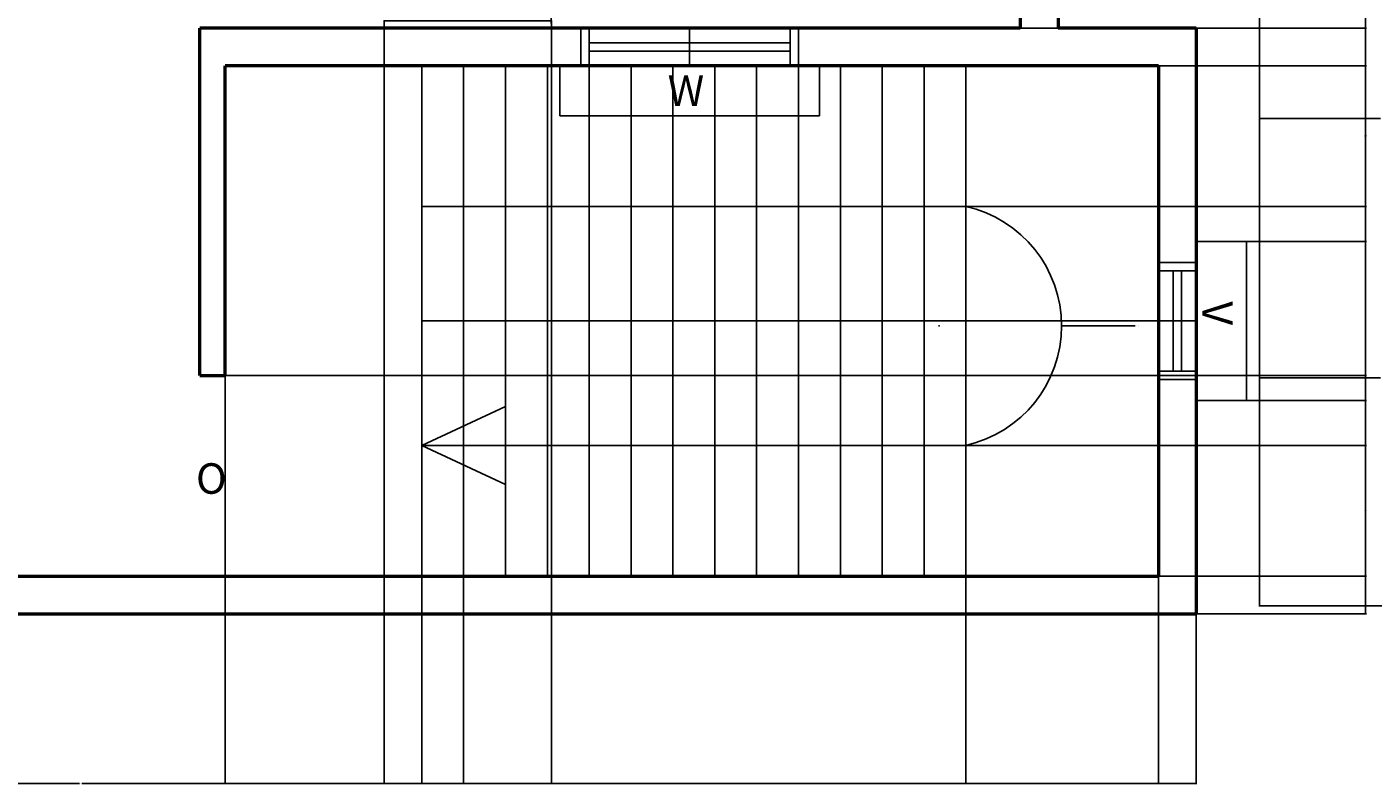
# Model space of a CAD drawing. Units: inches. Extents: x -73 to 1162, y -188 to 590.
# Tile 4 of 9: x 222 to 543, y -188 to -8. Entities that reach past the tile are written whole.
import ezdxf

# ---------------------------------------------------------------- set-up
doc = ezdxf.new("R2010")
doc.units = ezdxf.units.IN
doc.header["$MEASUREMENT"] = 0
for name, color, linetype, lineweight in [('A-ANNO-DIMS', 2, 'Continuous', 18), ('A-ANNO-TEXT', 7, 'Continuous', 25), ('A-DOOR', 3, 'Continuous', 25), ('A-FLOR-STRS', 3, 'Continuous', 25), ('A-GLAZ', 4, 'Continuous', 25), ('A-WALL', 7, 'Continuous', 50)]:
    doc.layers.add(name, color=color, linetype=linetype, lineweight=lineweight)
doc.styles.get("Standard").update_dxf_attribs({"font": 'arial.ttf'})
doc.dimstyles.get("Standard").update_dxf_attribs({"dimtxt": 0.18, "dimasz": 0.18, "dimexe": 0.18, "dimexo": 0.0625, "dimgap": 0.09, "dimtad": 0, "dimtih": 1, "dimtoh": 1, "dimdec": 1, "dimzin": 0, "dimdsep": 46, "dimlunit": 4, "dimtxsty": 'Standard', "dimcen": 0.09, "dimadec": 0, "dimazin": 0, "dimtfac": 1, "dimtdec": 1, "dimtofl": 0, "dimtmove": 0, "dimatfit": 3, "dimfxl": 1, "dimtolj": 1, "dimtzin": 0, "dimarcsym": 0})

# ---------------------------------------------------------------- blocks, each defined once
blk = doc.blocks.new('*U7')
for p, q in [((0, 0), (0, 6)), ((40, 0), (40, 6))]:
    blk.add_line(p, q)
blk.add_lwpolyline([(0, 0), (0, -40), (1.75, -40), (1.75, 0)], close=True)
blk.add_arc((0, 0), 40, 270, 360)
blk = doc.blocks.new('VENT-V')
for p, q in [((0, 9), (0, 21)), ((38, 21), (0, 21)), ((38, 9), (38, 21)), ((5, 9), (0, 9)), ((5, 0), (5, 9)), ((33, 0), (33, 9)), ((33, 9), (38, 9))]:
    blk.add_line(p, q)
blk = doc.blocks.new('*D58')
at = {"layer": 'A-ANNO-DIMS', "color": 0, "lineweight": -2, "transparency": 16777216}
for p, q in [((-31.83, -147.88), (-31.83, -188.5)), ((501.17, -147.88), (501.17, -188.5)), ((-31.65, -188.32), (234.38, -188.32)), ((500.99, -188.32), (234.96, -188.32))]:
    blk.add_line(p, q, dxfattribs=at)
at = {"layer": 'A-ANNO-DIMS', "color": 0, "transparency": 16777216}
for points in [[(-31.65, -188.29), (-31.65, -188.35), (-31.83, -188.32)], [(500.99, -188.29), (500.99, -188.35), (501.17, -188.32)]]:
    blk.add_solid(points, dxfattribs=at)
at = {"layer": 'Defpoints', "color": 0, "transparency": 16777216}
for p in [(-31.83, -147.82), (501.17, -147.82), (501.17, -188.32)]:
    blk.add_point(p, dxfattribs=at)
at = {"layer": 'A-ANNO-DIMS', "color": 0, "transparency": 16777216, "insert": (234.67, -188.32), "char_height": 0.18, "attachment_point": 5}
blk.add_mtext('\\A1;533', dxfattribs=at)
blk = doc.blocks.new('*D74')
at = {"layer": 'A-ANNO-DIMS', "color": 0, "lineweight": -2, "transparency": 16777216}
for p, q in [((480.23, 36.68), (541.85, 36.68)), ((541.67, 36.5), (541.67, 14.62)), ((541.67, -7.64), (541.67, 14.25)), ((501.23, -7.82), (541.85, -7.82))]:
    blk.add_line(p, q, dxfattribs=at)
at = {"layer": 'A-ANNO-DIMS', "color": 0, "transparency": 16777216}
for points in [[(541.64, 36.5), (541.7, 36.5), (541.67, 36.68)], [(541.64, -7.64), (541.7, -7.64), (541.67, -7.82)]]:
    blk.add_solid(points, dxfattribs=at)
at = {"layer": 'Defpoints', "color": 0, "transparency": 16777216}
for p in [(480.17, 36.68), (501.17, -7.82), (541.67, -7.82)]:
    blk.add_point(p, dxfattribs=at)
at = {"layer": 'A-ANNO-DIMS', "color": 0, "transparency": 16777216, "insert": (541.67, 14.43), "char_height": 0.18, "attachment_point": 5}
blk.add_mtext('\\A1;44.5', dxfattribs=at)
blk = doc.blocks.new('*D75')
at = {"layer": 'A-ANNO-DIMS', "color": 0, "lineweight": -2, "transparency": 16777216}
for p, q in [((501.23, -7.82), (541.85, -7.82)), ((541.67, -8), (541.67, -33.13)), ((541.67, -58.64), (541.67, -33.5)), ((501.23, -58.82), (541.85, -58.82))]:
    blk.add_line(p, q, dxfattribs=at)
at = {"layer": 'A-ANNO-DIMS', "color": 0, "transparency": 16777216}
for points in [[(541.64, -8), (541.7, -8), (541.67, -7.82)], [(541.64, -58.64), (541.7, -58.64), (541.67, -58.82)]]:
    blk.add_solid(points, dxfattribs=at)
at = {"layer": 'Defpoints', "color": 0, "transparency": 16777216}
for p in [(501.17, -7.82), (501.17, -58.82), (541.67, -58.82)]:
    blk.add_point(p, dxfattribs=at)
at = {"layer": 'A-ANNO-DIMS', "color": 0, "transparency": 16777216, "insert": (541.67, -33.32), "char_height": 0.18, "attachment_point": 5}
blk.add_mtext('\\A1;51', dxfattribs=at)
blk = doc.blocks.new('*D76')
at = {"layer": 'A-ANNO-DIMS', "color": 0, "lineweight": -2, "transparency": 16777216}
for p, q in [((501.23, -96.82), (541.85, -96.82)), ((541.67, -97), (541.67, -122.13)), ((541.67, -147.64), (541.67, -122.5)), ((501.23, -147.82), (541.85, -147.82))]:
    blk.add_line(p, q, dxfattribs=at)
at = {"layer": 'A-ANNO-DIMS', "color": 0, "transparency": 16777216}
for points in [[(541.64, -97), (541.7, -97), (541.67, -96.82)], [(541.64, -147.64), (541.7, -147.64), (541.67, -147.82)]]:
    blk.add_solid(points, dxfattribs=at)
at = {"layer": 'Defpoints', "color": 0, "transparency": 16777216}
for p in [(501.17, -96.82), (501.17, -147.82), (541.67, -147.82)]:
    blk.add_point(p, dxfattribs=at)
at = {"layer": 'A-ANNO-DIMS', "color": 0, "transparency": 16777216, "insert": (541.67, -122.32), "char_height": 0.18, "attachment_point": 5}
blk.add_mtext('\\A1;51', dxfattribs=at)
blk = doc.blocks.new('*D77')
at = {"layer": 'A-ANNO-DIMS', "color": 0, "lineweight": -2, "transparency": 16777216}
for p, q in [((269.17, -16.88), (269.17, -188.5)), ((316.17, -16.88), (316.17, -188.5)), ((269.35, -188.32), (292.45, -188.32)), ((315.99, -188.32), (292.89, -188.32))]:
    blk.add_line(p, q, dxfattribs=at)
at = {"layer": 'A-ANNO-DIMS', "color": 0, "transparency": 16777216}
for points in [[(269.35, -188.29), (269.35, -188.35), (269.17, -188.32)], [(315.99, -188.29), (315.99, -188.35), (316.17, -188.32)]]:
    blk.add_solid(points, dxfattribs=at)
at = {"layer": 'Defpoints', "color": 0, "transparency": 16777216}
for p in [(269.17, -16.82), (316.17, -16.82), (316.17, -188.32)]:
    blk.add_point(p, dxfattribs=at)
at = {"layer": 'A-ANNO-DIMS', "color": 0, "transparency": 16777216, "insert": (292.67, -188.32), "char_height": 0.18, "attachment_point": 5}
blk.add_mtext('\\A1;47', dxfattribs=at)
blk = doc.blocks.new('*D78')
at = {"layer": 'A-ANNO-DIMS', "color": 0, "lineweight": -2, "transparency": 16777216}
for p, q in [((316.17, -16.88), (316.17, -188.5)), ((326.17, -16.88), (326.17, -188.5)), ((316.35, -188.32), (320.96, -188.32)), ((325.99, -188.32), (321.38, -188.32))]:
    blk.add_line(p, q, dxfattribs=at)
at = {"layer": 'A-ANNO-DIMS', "color": 0, "transparency": 16777216}
for points in [[(316.35, -188.29), (316.35, -188.35), (316.17, -188.32)], [(325.99, -188.29), (325.99, -188.35), (326.17, -188.32)]]:
    blk.add_solid(points, dxfattribs=at)
at = {"layer": 'Defpoints', "color": 0, "transparency": 16777216}
for p in [(316.17, -16.82), (326.17, -16.82), (326.17, -188.32)]:
    blk.add_point(p, dxfattribs=at)
at = {"layer": 'A-ANNO-DIMS', "color": 0, "transparency": 16777216, "insert": (321.17, -188.32), "char_height": 0.18, "attachment_point": 5}
blk.add_mtext('\\A1;10', dxfattribs=at)
blk = doc.blocks.new('*D79')
at = {"layer": 'A-ANNO-DIMS', "color": 0, "lineweight": -2, "transparency": 16777216}
for p, q in [((326.17, -16.88), (326.17, -188.5)), ((446.17, -16.88), (446.17, -188.5)), ((326.35, -188.32), (385.89, -188.32)), ((445.99, -188.32), (386.45, -188.32))]:
    blk.add_line(p, q, dxfattribs=at)
at = {"layer": 'A-ANNO-DIMS', "color": 0, "transparency": 16777216}
for points in [[(326.35, -188.29), (326.35, -188.35), (326.17, -188.32)], [(445.99, -188.29), (445.99, -188.35), (446.17, -188.32)]]:
    blk.add_solid(points, dxfattribs=at)
at = {"layer": 'Defpoints', "color": 0, "transparency": 16777216}
for p in [(326.17, -16.82), (446.17, -16.82), (446.17, -188.32)]:
    blk.add_point(p, dxfattribs=at)
at = {"layer": 'A-ANNO-DIMS', "color": 0, "transparency": 16777216, "insert": (386.17, -188.32), "char_height": 0.18, "attachment_point": 5}
blk.add_mtext('\\A1;120', dxfattribs=at)
blk = doc.blocks.new('*D80')
at = {"layer": 'A-ANNO-DIMS', "color": 0, "lineweight": -2, "transparency": 16777216}
for p, q in [((446.17, -16.88), (446.17, -188.5)), ((492.17, -16.88), (492.17, -188.5)), ((446.35, -188.32), (468.95, -188.32)), ((491.99, -188.32), (469.39, -188.32))]:
    blk.add_line(p, q, dxfattribs=at)
at = {"layer": 'A-ANNO-DIMS', "color": 0, "transparency": 16777216}
for points in [[(446.35, -188.29), (446.35, -188.35), (446.17, -188.32)], [(491.99, -188.29), (491.99, -188.35), (492.17, -188.32)]]:
    blk.add_solid(points, dxfattribs=at)
at = {"layer": 'Defpoints', "color": 0, "transparency": 16777216}
for p in [(446.17, -16.82), (492.17, -16.82), (492.17, -188.32)]:
    blk.add_point(p, dxfattribs=at)
at = {"layer": 'A-ANNO-DIMS', "color": 0, "transparency": 16777216, "insert": (469.17, -188.32), "char_height": 0.18, "attachment_point": 5}
blk.add_mtext('\\A1;46', dxfattribs=at)
blk = doc.blocks.new('*D81')
at = {"layer": 'A-ANNO-DIMS', "color": 0, "lineweight": -2, "transparency": 16777216}
for p, q in [((263.23, -7.82), (541.85, -7.82)), ((541.67, -8), (541.67, -49.13)), ((541.67, -90.64), (541.67, -49.5)), ((263.23, -90.82), (541.85, -90.82))]:
    blk.add_line(p, q, dxfattribs=at)
at = {"layer": 'A-ANNO-DIMS', "color": 0, "transparency": 16777216}
for points in [[(541.64, -8), (541.7, -8), (541.67, -7.82)], [(541.64, -90.64), (541.7, -90.64), (541.67, -90.82)]]:
    blk.add_solid(points, dxfattribs=at)
at = {"layer": 'Defpoints', "color": 0, "transparency": 16777216}
for p in [(263.17, -7.82), (541.67, -7.82), (263.17, -90.82)]:
    blk.add_point(p, dxfattribs=at)
at = {"layer": 'A-ANNO-DIMS', "color": 0, "transparency": 16777216, "insert": (541.67, -49.32), "char_height": 0.18, "attachment_point": 5}
blk.add_mtext('\\A1;83', dxfattribs=at)
blk = doc.blocks.new('*D82')
at = {"layer": 'A-ANNO-DIMS', "color": 0, "lineweight": -2, "transparency": 16777216}
for p, q in [((446.23, -16.82), (541.85, -16.82)), ((541.67, -17), (541.67, -33.45)), ((541.67, -50.27), (541.67, -33.82)), ((446.23, -50.45), (541.85, -50.45))]:
    blk.add_line(p, q, dxfattribs=at)
at = {"layer": 'A-ANNO-DIMS', "color": 0, "transparency": 16777216}
for points in [[(541.64, -17), (541.7, -17), (541.67, -16.82)], [(541.64, -50.27), (541.7, -50.27), (541.67, -50.45)]]:
    blk.add_solid(points, dxfattribs=at)
at = {"layer": 'Defpoints', "color": 0, "transparency": 16777216}
for p in [(446.17, -16.82), (446.17, -50.45), (541.67, -50.45)]:
    blk.add_point(p, dxfattribs=at)
at = {"layer": 'A-ANNO-DIMS', "color": 0, "transparency": 16777216, "insert": (541.67, -33.63), "char_height": 0.18, "attachment_point": 5}
blk.add_mtext('\\A1;33.636', dxfattribs=at)
blk = doc.blocks.new('*D83')
at = {"layer": 'A-ANNO-DIMS', "color": 0, "lineweight": -2, "transparency": 16777216}
for p, q in [((446.23, -50.45), (541.85, -50.45)), ((541.67, -50.63), (541.67, -78.82)), ((541.67, -107.37), (541.67, -79.18)), ((446.23, -107.55), (541.85, -107.55))]:
    blk.add_line(p, q, dxfattribs=at)
at = {"layer": 'A-ANNO-DIMS', "color": 0, "transparency": 16777216}
for points in [[(541.64, -50.63), (541.7, -50.63), (541.67, -50.45)], [(541.64, -107.37), (541.7, -107.37), (541.67, -107.55)]]:
    blk.add_solid(points, dxfattribs=at)
at = {"layer": 'Defpoints', "color": 0, "transparency": 16777216}
for p in [(446.17, -50.45), (446.17, -107.55), (541.67, -107.55)]:
    blk.add_point(p, dxfattribs=at)
at = {"layer": 'A-ANNO-DIMS', "color": 0, "transparency": 16777216, "insert": (541.67, -79), "char_height": 0.18, "attachment_point": 5}
blk.add_mtext('\\A1;57.1', dxfattribs=at)
blk = doc.blocks.new('*D84')
at = {"layer": 'A-ANNO-DIMS', "color": 0, "lineweight": -2, "transparency": 16777216}
for p, q in [((446.23, -107.55), (541.85, -107.55)), ((541.67, -107.73), (541.67, -123)), ((541.67, -138.64), (541.67, -123.36)), ((446.23, -138.82), (541.85, -138.82))]:
    blk.add_line(p, q, dxfattribs=at)
at = {"layer": 'A-ANNO-DIMS', "color": 0, "transparency": 16777216}
for points in [[(541.64, -107.73), (541.7, -107.73), (541.67, -107.55)], [(541.64, -138.64), (541.7, -138.64), (541.67, -138.82)]]:
    blk.add_solid(points, dxfattribs=at)
at = {"layer": 'Defpoints', "color": 0, "transparency": 16777216}
for p in [(446.17, -107.55), (446.17, -138.82), (541.67, -138.82)]:
    blk.add_point(p, dxfattribs=at)
at = {"layer": 'A-ANNO-DIMS', "color": 0, "transparency": 16777216, "insert": (541.67, -123.18), "char_height": 0.18, "attachment_point": 5}
blk.add_mtext('\\A1;31.27', dxfattribs=at)
blk = doc.blocks.new('*D85')
at = {"layer": 'A-ANNO-DIMS', "color": 0, "lineweight": -2, "transparency": 16777216}
for p, q in [((307.17, -7.88), (307.17, -188.5)), ((347.17, -7.88), (347.17, -188.5)), ((307.35, -188.32), (326.95, -188.32)), ((346.99, -188.32), (327.39, -188.32))]:
    blk.add_line(p, q, dxfattribs=at)
at = {"layer": 'A-ANNO-DIMS', "color": 0, "transparency": 16777216}
for points in [[(307.35, -188.29), (307.35, -188.35), (307.17, -188.32)], [(346.99, -188.29), (346.99, -188.35), (347.17, -188.32)]]:
    blk.add_solid(points, dxfattribs=at)
at = {"layer": 'Defpoints', "color": 0, "transparency": 16777216}
for p in [(307.17, -7.82), (347.17, -7.82), (347.17, -188.32)]:
    blk.add_point(p, dxfattribs=at)
at = {"layer": 'A-ANNO-DIMS', "color": 0, "transparency": 16777216, "insert": (327.17, -188.32), "char_height": 0.18, "attachment_point": 5}
blk.add_mtext('\\A1;40', dxfattribs=at)
blk = doc.blocks.new('*D104')
at = {"layer": 'A-ANNO-DIMS', "color": 0, "lineweight": -2, "transparency": 16777216}
for p, q in [((557.24, 154.09), (516.13, 154.09)), ((516.31, 153.91), (516.31, 4.27)), ((516.31, -145.73), (516.31, 3.91)), ((557.24, -145.91), (516.13, -145.91))]:
    blk.add_line(p, q, dxfattribs=at)
at = {"layer": 'A-ANNO-DIMS', "color": 0, "transparency": 16777216}
for points in [[(516.28, 153.91), (516.34, 153.91), (516.31, 154.09)], [(516.28, -145.73), (516.34, -145.73), (516.31, -145.91)]]:
    blk.add_solid(points, dxfattribs=at)
at = {"layer": 'Defpoints', "color": 0, "transparency": 16777216}
for p in [(557.31, 154.09), (516.31, -145.91), (557.31, -145.91)]:
    blk.add_point(p, dxfattribs=at)
at = {"layer": 'A-ANNO-DIMS', "color": 0, "transparency": 16777216, "insert": (516.31, 4.09), "char_height": 0.18, "attachment_point": 5}
blk.add_mtext('\\A1;300', dxfattribs=at)
blk = doc.blocks.new('*D106')
at = {"layer": 'A-ANNO-DIMS', "color": 0, "lineweight": -2, "transparency": 16777216}
for p, q in [((545.24, 54.09), (516.13, 54.09)), ((516.31, 53.91), (516.31, 12.52)), ((516.31, -29.23), (516.31, 12.16)), ((545.24, -29.41), (516.13, -29.41))]:
    blk.add_line(p, q, dxfattribs=at)
at = {"layer": 'A-ANNO-DIMS', "color": 0, "transparency": 16777216}
for points in [[(516.28, 53.91), (516.34, 53.91), (516.31, 54.09)], [(516.28, -29.23), (516.34, -29.23), (516.31, -29.41)]]:
    blk.add_solid(points, dxfattribs=at)
at = {"layer": 'Defpoints', "color": 0, "transparency": 16777216}
for p in [(545.31, 54.09), (516.31, -29.41), (545.31, -29.41)]:
    blk.add_point(p, dxfattribs=at)
at = {"layer": 'A-ANNO-DIMS', "color": 0, "transparency": 16777216, "insert": (516.31, 12.34), "char_height": 0.18, "attachment_point": 5}
blk.add_mtext('\\A1;83.5', dxfattribs=at)
blk = doc.blocks.new('*D107')
at = {"layer": 'A-ANNO-DIMS', "color": 0, "lineweight": -2, "transparency": 16777216}
for p, q in [((545.24, -91.41), (516.13, -91.41)), ((516.31, -91.59), (516.31, -118.48)), ((516.31, -145.73), (516.31, -118.84)), ((557.24, -145.91), (516.13, -145.91))]:
    blk.add_line(p, q, dxfattribs=at)
at = {"layer": 'A-ANNO-DIMS', "color": 0, "transparency": 16777216}
for points in [[(516.28, -91.59), (516.34, -91.59), (516.31, -91.41)], [(516.28, -145.73), (516.34, -145.73), (516.31, -145.91)]]:
    blk.add_solid(points, dxfattribs=at)
at = {"layer": 'Defpoints', "color": 0, "transparency": 16777216}
for p in [(545.31, -91.41), (516.31, -145.91), (557.31, -145.91)]:
    blk.add_point(p, dxfattribs=at)
at = {"layer": 'A-ANNO-DIMS', "color": 0, "transparency": 16777216, "insert": (516.31, -118.66), "char_height": 0.18, "attachment_point": 5}
blk.add_mtext('\\A1;54.5', dxfattribs=at)
blk = doc.blocks.new('*D161')
at = {"layer": 'A-ANNO-DIMS', "color": 0, "lineweight": -2, "transparency": 16777216}
for p, q in [((439.66, -79), (439.84, -79)), ((439.75, -79.09), (439.75, -78.91)), ((486.57, -79), (469.19, -79))]:
    blk.add_line(p, q, dxfattribs=at)
at = {"layer": 'A-ANNO-DIMS', "color": 0, "transparency": 16777216}
blk.add_solid([(469.19, -78.97), (469.19, -79.03), (469.01, -79)], dxfattribs=at)
at = {"layer": 'Defpoints', "color": 0, "transparency": 16777216}
for p in [(439.75, -79), (469.01, -79)]:
    blk.add_point(p, dxfattribs=at)
at = {"layer": 'A-ANNO-DIMS', "color": 0, "transparency": 16777216, "insert": (487.05, -79), "char_height": 0.18, "attachment_point": 5}
blk.add_mtext('\\A1;R29.26', dxfattribs=at)

msp = doc.modelspace()

# ---------------------------------------------------------------- linework, layer by layer
at = {"layer": 'A-FLOR-STRS'}
for p, q in [((316.17, -16.8156), (316.17, -138.8156)), ((326.17, -16.8156), (326.17, -138.8156)), ((336.17, -16.8156), (336.17, -138.8156)), ((346.17, -16.8156), (346.17, -138.8156)), ((356.17, -16.8156), (356.17, -138.8156)), ((366.17, -16.8156), (366.17, -138.8156)), ((376.17, -16.8156), (376.17, -138.8156)), ((386.17, -16.8156), (386.17, -138.8156)), ((396.17, -16.8156), (396.17, -138.8156)), ((406.17, -16.8156), (406.17, -138.8156)), ((416.17, -16.8156), (416.17, -138.8156)), ((426.17, -16.8156), (426.17, -138.8156)), ((436.17, -16.8156), (436.17, -138.8156)), ((446.17, -16.8156), (446.17, -138.8156)), ((446.17, -50.4515), (316.17, -50.4515)), ((316.17, -77.8156), (492.17, -77.8156)), ((316.17, -107.5469), (336.17, -98.2298)), ((446.17, -107.5469), (316.17, -107.5469)), ((316.17, -107.5469), (336.17, -116.864))]:
    msp.add_line(p, q, dxfattribs=at)
msp.add_arc((439.7494, -78.9992), 29.2608, 282.675347, 77.324653, dxfattribs=at)
at = {"layer": 'A-GLAZ'}
for p, q in [((354.17, -7.8156), (354.17, -16.8156)), ((356.17, -7.8156), (356.17, -16.8156)), ((380.17, -7.8156), (380.1411, -16.8155)), ((380.17, -7.8156), (380.17, -16.8156)), ((404.17, -7.8156), (404.17, -16.8156)), ((406.17, -7.8156), (406.17, -16.8156)), ((404.17, -11.3156), (356.17, -11.3156)), ((404.17, -13.3156), (356.17, -13.3156)), ((354.17, -16.8156), (349.17, -16.8156)), ((349.17, -16.8156), (349.17, -28.8156)), ((406.17, -16.8156), (411.17, -16.8156)), ((411.17, -16.8156), (411.17, -28.8156)), ((411.17, -28.8156), (349.17, -28.8156)), ((492.17, -65.8156), (501.17, -65.8156)), ((495.67, -65.8156), (495.67, -89.8156)), ((497.67, -65.8156), (497.67, -89.8156)), ((492.17, -77.8156), (501.17, -77.8156)), ((492.17, -89.8156), (501.17, -89.8156))]:
    msp.add_line(p, q, dxfattribs=at)
at = {"layer": 'A-WALL'}
for p, q in [((468.17, 152.1844), (468.17, -7.8156)), ((459.17, 143.1844), (459.17, -7.8156)), ((263.17, -90.8156), (263.17, -7.8156)), ((301.17, -7.8156), (263.17, -7.8156)), ((459.17, -7.8156), (301.17, -7.8156)), ((501.17, -7.8156), (468.17, -7.8156)), ((501.17, -7.8156), (501.17, -147.8156)), ((492.17, -16.8156), (269.17, -16.8156)), ((269.17, -90.8156), (269.17, -16.8156)), ((492.17, -16.8156), (492.17, -138.8156)), ((263.17, -90.8156), (269.17, -90.8156)), ((218.6031, -138.8156), (316.17, -138.8156)), ((269.17, -138.8156), (492.17, -138.8156)), ((218.6031, -147.8156), (501.17, -147.8156))]:
    msp.add_line(p, q, dxfattribs=at)

# ---------------------------------------------------------------- block references
at = {"layer": 'A-DOOR', "rotation": 90}
msp.add_blockref('*U7', (307.17, -7.8156), dxfattribs=at)
at = {"layer": 'A-GLAZ', "rotation": 270.0000000000003}
msp.add_blockref('VENT-V', (492.1696, -58.8156), dxfattribs=at)

# ---------------------------------------------------------------- texts
at = {"layer": 'A-ANNO-TEXT'}
for s, p in [('W', (374.9183, -26.4009)), ('O', (262.2216, -119.1099))]:
    msp.add_text(s, height=7.2829, dxfattribs=at).set_placement(p)
msp.add_text('V', height=7.2829, rotation=270, dxfattribs=at).set_placement((502.6305, -73.1122))

# ---------------------------------------------------------------- dimensions: what is measured, and where the dimension line sits
at = {"layer": 'A-ANNO-DIMS'}
for base, p1, p2, override, picture, middle in [((516.307, -145.9077), (557.307, 154.0923), (557.307, -145.9077), {"dimdec": 0, "dimlfac": 1, "dimrnd": 0, "dimzin": 0, "dimdsep": 46, "dimlunit": 2}, '*D104', (516.307, 4.0923)), ((516.307, -29.4077), (545.307, 54.0923), (545.307, -29.4077), {"dimdec": 1, "dimlfac": 1, "dimrnd": 0, "dimzin": 0, "dimdsep": 46, "dimlunit": 2}, '*D106', (516.307, 12.3423)), ((541.67, -7.8156), (480.17, 36.6844), (501.17, -7.8156), {"dimdec": 1, "dimlfac": 1, "dimrnd": 0, "dimzin": 0, "dimdsep": 46, "dimlunit": 2}, '*D74', (541.67, 14.4344)), ((541.67, -7.8156), (263.17, -90.8156), (263.17, -7.8156), {"dimdec": 0, "dimlfac": 1, "dimrnd": 0, "dimzin": 0, "dimdsep": 46, "dimlunit": 2}, '*D81', (541.67, -49.3156)), ((541.67, -58.8156), (501.17, -7.8156), (501.17, -58.8156), {"dimdec": 0, "dimlfac": 1, "dimrnd": 0, "dimzin": 0, "dimdsep": 46, "dimlunit": 2}, '*D75', (541.67, -33.3156)), ((541.67, -50.4515), (446.17, -16.8156), (446.17, -50.4515), {"dimdec": 3, "dimlfac": 1, "dimrnd": 0, "dimzin": 0, "dimdsep": 46, "dimlunit": 2}, '*D82', (541.67, -33.6335)), ((541.67, -107.5469), (446.17, -50.4515), (446.17, -107.5469), {"dimdec": 1, "dimlfac": 1, "dimrnd": 0, "dimzin": 0, "dimdsep": 46, "dimlunit": 2}, '*D83', (541.67, -78.9992)), ((516.307, -145.9077), (545.307, -91.4077), (557.307, -145.9077), {"dimdec": 1, "dimlfac": 1, "dimrnd": 0, "dimzin": 0, "dimdsep": 46, "dimlunit": 2}, '*D107', (516.307, -118.6577)), ((541.67, -147.8156), (501.17, -96.8156), (501.17, -147.8156), {"dimdec": 0, "dimlfac": 1, "dimrnd": 0, "dimzin": 0, "dimdsep": 46, "dimlunit": 2}, '*D76', (541.67, -122.3156)), ((541.67, -138.8156), (446.17, -107.5469), (446.17, -138.8156), {"dimdec": 2, "dimlfac": 1, "dimrnd": 0, "dimzin": 0, "dimdsep": 46, "dimlunit": 2}, '*D84', (541.67, -123.1812))]:
    dim = msp.add_linear_dim(base=base, p1=p1, p2=p2, angle=90, dimstyle='Standard', override=override, dxfattribs=at)
    dim.commit()
    dim.dimension.update_dxf_attribs({"geometry": picture, "text_midpoint": middle})
for base, p1, p2, picture, middle in [((347.17, -188.3156), (307.17, -7.8156), (347.17, -7.8156), '*D85', (327.17, -188.3156)), ((316.17, -188.3156), (269.17, -16.8156), (316.17, -16.8156), '*D77', (292.67, -188.3156)), ((326.17, -188.3156), (316.17, -16.8156), (326.17, -16.8156), '*D78', (321.17, -188.3156)), ((446.17, -188.3156), (326.17, -16.8156), (446.17, -16.8156), '*D79', (386.17, -188.3156)), ((492.17, -188.3156), (446.17, -16.8156), (492.17, -16.8156), '*D80', (469.17, -188.3156)), ((501.17, -188.3156), (-31.83, -147.8156), (501.17, -147.8156), '*D58', (234.67, -188.3156))]:
    dim = msp.add_linear_dim(base=base, p1=p1, p2=p2, dimstyle='Standard', override={"dimdec": 0, "dimlfac": 1, "dimrnd": 0, "dimzin": 0, "dimdsep": 46, "dimlunit": 2}, dxfattribs=at)
    dim.commit()
    dim.dimension.update_dxf_attribs({"geometry": picture, "text_midpoint": middle})
dim = msp.add_radius_dim(center=(439.7494, -78.9992), mpoint=(469.0102, -79), dimstyle='Standard', override={"dimdec": 2, "dimlfac": 1, "dimrnd": 0, "dimzin": 0, "dimdsep": 46, "dimlunit": 2}, dxfattribs=at)
dim.commit()
dim.dimension.update_dxf_attribs({"geometry": '*D161', "text_midpoint": (486.5667, -79.0005), "dimtype": 164})

doc.saveas('drawing.dxf')
